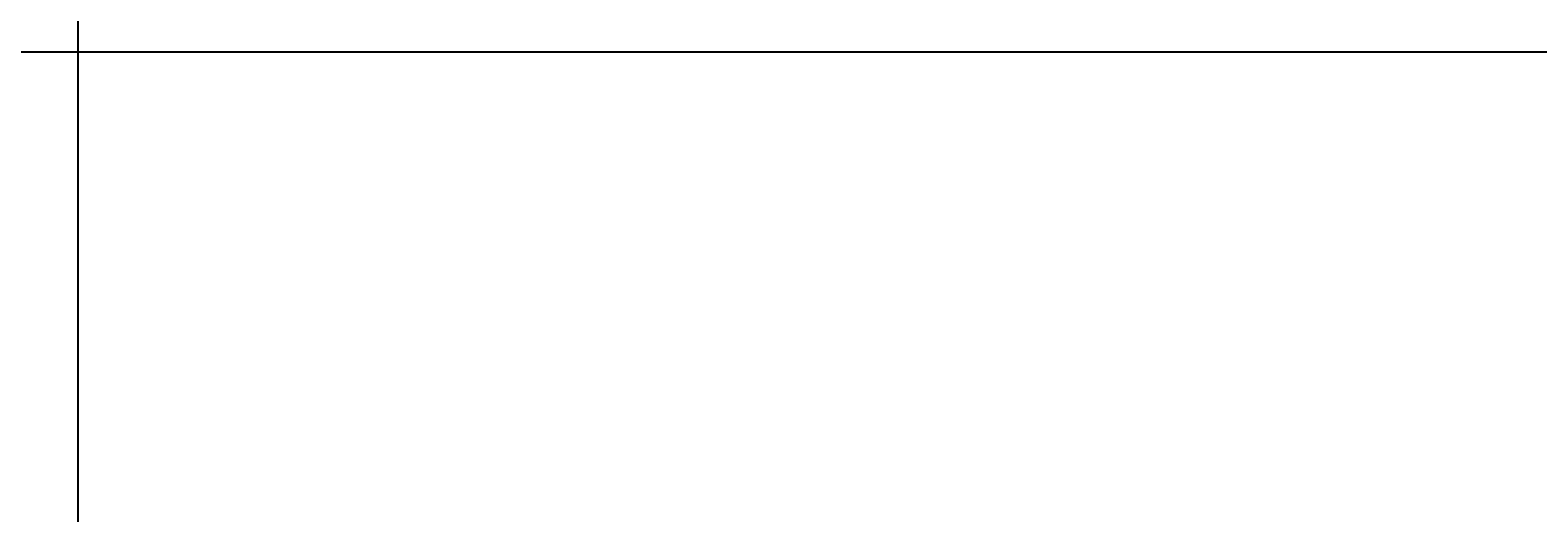
# Model space of a CAD drawing. Units: inches. Extents: x 35362 to 73946, y 43607 to 67532.
# Tile 98 of 134: x 50119 to 50761, y 49064 to 49269. Entities that reach past the tile are written whole.
import ezdxf

# ---------------------------------------------------------------- set-up
doc = ezdxf.new("R2010")
doc.units = ezdxf.units.IN
doc.header["$MEASUREMENT"] = 0
doc.layers.add('A-ANNO-DIMS', color=2, linetype='Continuous', lineweight=18)
doc.styles.get("Standard").update_dxf_attribs({"font": 'arial.ttf'})
doc.dimstyles.get("Standard").update_dxf_attribs({"dimtxt": 0.18, "dimasz": 0.18, "dimexe": 0.18, "dimexo": 0.0625, "dimgap": 0.09, "dimtad": 0, "dimtih": 1, "dimtoh": 1, "dimdec": 4, "dimzin": 0, "dimdsep": 46, "dimtxsty": 'Standard', "dimcen": 0.09, "dimadec": 0, "dimazin": 0, "dimtfac": 1, "dimtdec": 4, "dimtofl": 0, "dimtmove": 0, "dimatfit": 3, "dimfxl": 1, "dimtolj": 1, "dimtzin": 0, "dimarcsym": 0})

# ---------------------------------------------------------------- blocks, each defined once
blk = doc.blocks.new('*D11')
at = {"layer": 'A-ANNO-DIMS', "color": 0, "lineweight": -2, "transparency": 16777216}
for p, q in [((47978.66, 56028.77), (47978.66, 43606.68)), ((53109.76, 56028.77), (53109.76, 43606.68)), ((47978.84, 43606.86), (50543.87, 43606.86)), ((53109.58, 43606.86), (50544.55, 43606.86))]:
    blk.add_line(p, q, dxfattribs=at)
at = {"layer": 'A-ANNO-DIMS', "color": 0, "transparency": 16777216}
for points in [[(47978.84, 43606.89), (47978.84, 43606.83), (47978.66, 43606.86)], [(53109.58, 43606.89), (53109.58, 43606.83), (53109.76, 43606.86)]]:
    blk.add_solid(points, dxfattribs=at)
at = {"layer": 'Defpoints', "color": 0, "transparency": 16777216}
for p in [(47978.66, 56028.84), (53109.76, 56028.84), (53109.76, 43606.86)]:
    blk.add_point(p, dxfattribs=at)
at = {"layer": 'A-ANNO-DIMS', "color": 0, "transparency": 16777216, "insert": (50544.21, 43606.86), "char_height": 0.18, "attachment_point": 5}
blk.add_mtext('\\A1;5131', dxfattribs=at)
blk = doc.blocks.new('*D13')
at = {"layer": 'A-ANNO-DIMS', "color": 0, "lineweight": -2, "transparency": 16777216}
for p, q in [((48373.49, 51694.02), (48373.49, 43606.68)), ((51029.04, 51694.02), (51029.04, 43606.68)), ((48373.67, 43606.86), (49700.8, 43606.86)), ((51028.86, 43606.86), (49701.73, 43606.86))]:
    blk.add_line(p, q, dxfattribs=at)
at = {"layer": 'A-ANNO-DIMS', "color": 0, "transparency": 16777216}
for points in [[(48373.67, 43606.89), (48373.67, 43606.83), (48373.49, 43606.86)], [(51028.86, 43606.89), (51028.86, 43606.83), (51029.04, 43606.86)]]:
    blk.add_solid(points, dxfattribs=at)
at = {"layer": 'Defpoints', "color": 0, "transparency": 16777216}
for p in [(48373.49, 51694.09), (51029.04, 51694.09), (51029.04, 43606.86)]:
    blk.add_point(p, dxfattribs=at)
at = {"layer": 'A-ANNO-DIMS', "color": 0, "transparency": 16777216, "insert": (49701.27, 43606.86), "char_height": 0.18, "attachment_point": 5}
blk.add_mtext('\\A1;2655.6', dxfattribs=at)
blk = doc.blocks.new('*D17')
at = {"layer": 'A-ANNO-DIMS', "color": 0, "lineweight": -2, "transparency": 16777216}
for p, q in [((49923.31, 61293.22), (49923.31, 43606.68)), ((51913.93, 61293.22), (51913.93, 43606.68)), ((49923.49, 43606.86), (50918.16, 43606.86)), ((51913.75, 43606.86), (50919.07, 43606.86))]:
    blk.add_line(p, q, dxfattribs=at)
at = {"layer": 'A-ANNO-DIMS', "color": 0, "transparency": 16777216}
for points in [[(49923.49, 43606.89), (49923.49, 43606.83), (49923.31, 43606.86)], [(51913.75, 43606.89), (51913.75, 43606.83), (51913.93, 43606.86)]]:
    blk.add_solid(points, dxfattribs=at)
at = {"layer": 'Defpoints', "color": 0, "transparency": 16777216}
for p in [(49923.31, 61293.29), (51913.93, 61293.29), (51913.93, 43606.86)]:
    blk.add_point(p, dxfattribs=at)
at = {"layer": 'A-ANNO-DIMS', "color": 0, "transparency": 16777216, "insert": (50918.62, 43606.86), "char_height": 0.18, "attachment_point": 5}
blk.add_mtext('\\A1;1990.6', dxfattribs=at)
blk = doc.blocks.new('*D67')
at = {"layer": 'A-ANNO-DIMS', "color": 0, "lineweight": -2, "transparency": 16777216}
for p, q in [((56873.54, 53351.53), (35361.77, 53351.53)), ((35361.95, 53351.35), (35361.95, 49400.89)), ((35361.95, 45450.07), (35361.95, 49400.53)), ((53793.58, 45449.89), (35361.77, 45449.89))]:
    blk.add_line(p, q, dxfattribs=at)
at = {"layer": 'A-ANNO-DIMS', "color": 0, "transparency": 16777216}
for points in [[(35361.92, 53351.35), (35361.98, 53351.35), (35361.95, 53351.53)], [(35361.92, 45450.07), (35361.98, 45450.07), (35361.95, 45449.89)]]:
    blk.add_solid(points, dxfattribs=at)
at = {"layer": 'Defpoints', "color": 0, "transparency": 16777216}
for p in [(35361.95, 53351.53), (56873.6, 53351.53), (53793.64, 45449.89)]:
    blk.add_point(p, dxfattribs=at)
at = {"layer": 'A-ANNO-DIMS', "color": 0, "transparency": 16777216, "insert": (35361.95, 49400.71), "char_height": 0.18, "attachment_point": 5}
blk.add_mtext('\\A1;7901.6', dxfattribs=at)
blk = doc.blocks.new('*D84')
at = {"layer": 'A-ANNO-DIMS', "color": 0, "lineweight": -2, "transparency": 16777216}
for p, q in [((55540.23, 49259.94), (35361.77, 49259.94)), ((35361.95, 49259.76), (35361.95, 49115.14)), ((35361.95, 48970.16), (35361.95, 49114.78)), ((55540.23, 48969.98), (35361.77, 48969.98))]:
    blk.add_line(p, q, dxfattribs=at)
at = {"layer": 'A-ANNO-DIMS', "color": 0, "transparency": 16777216}
for points in [[(35361.92, 49259.76), (35361.98, 49259.76), (35361.95, 49259.94)], [(35361.92, 48970.16), (35361.98, 48970.16), (35361.95, 48969.98)]]:
    blk.add_solid(points, dxfattribs=at)
at = {"layer": 'Defpoints', "color": 0, "transparency": 16777216}
for p in [(35361.95, 49259.94), (55540.3, 49259.94), (55540.3, 48969.98)]:
    blk.add_point(p, dxfattribs=at)
at = {"layer": 'A-ANNO-DIMS', "color": 0, "transparency": 16777216, "insert": (35361.95, 49114.96), "char_height": 0.18, "attachment_point": 5}
blk.add_mtext('\\A1;289.96', dxfattribs=at)
blk = doc.blocks.new('*D86')
at = {"layer": 'A-ANNO-DIMS', "color": 0, "lineweight": -2, "transparency": 16777216}
for p, q in [((51285.53, 49320.08), (35361.77, 49320.08)), ((35361.95, 49319.9), (35361.95, 49120.26)), ((35361.95, 48920.26), (35361.95, 49119.9)), ((51285.53, 48920.08), (35361.77, 48920.08))]:
    blk.add_line(p, q, dxfattribs=at)
at = {"layer": 'A-ANNO-DIMS', "color": 0, "transparency": 16777216}
for points in [[(35361.92, 49319.9), (35361.98, 49319.9), (35361.95, 49320.08)], [(35361.92, 48920.26), (35361.98, 48920.26), (35361.95, 48920.08)]]:
    blk.add_solid(points, dxfattribs=at)
at = {"layer": 'Defpoints', "color": 0, "transparency": 16777216}
for p in [(35361.95, 49320.08), (51285.59, 49320.08), (51285.59, 48920.08)]:
    blk.add_point(p, dxfattribs=at)
at = {"layer": 'A-ANNO-DIMS', "color": 0, "transparency": 16777216, "insert": (35361.95, 49120.08), "char_height": 0.18, "attachment_point": 5}
blk.add_mtext('\\A1;400.0', dxfattribs=at)
blk = doc.blocks.new('*D107')
at = {"layer": 'A-ANNO-DIMS', "color": 0, "lineweight": -2, "transparency": 16777216}
for p, q in [((50139.56, 59850.01), (50139.56, 43606.68)), ((51320.81, 59850.01), (51320.81, 43606.68)), ((50139.74, 43606.86), (50729.73, 43606.86)), ((51320.63, 43606.86), (50730.64, 43606.86))]:
    blk.add_line(p, q, dxfattribs=at)
at = {"layer": 'A-ANNO-DIMS', "color": 0, "transparency": 16777216}
for points in [[(50139.74, 43606.89), (50139.74, 43606.83), (50139.56, 43606.86)], [(51320.63, 43606.89), (51320.63, 43606.83), (51320.81, 43606.86)]]:
    blk.add_solid(points, dxfattribs=at)
at = {"layer": 'Defpoints', "color": 0, "transparency": 16777216}
for p in [(50139.56, 59850.08), (51320.81, 59850.08), (51320.81, 43606.86)]:
    blk.add_point(p, dxfattribs=at)
at = {"layer": 'A-ANNO-DIMS', "color": 0, "transparency": 16777216, "insert": (50730.19, 43606.86), "char_height": 0.18, "attachment_point": 5}
blk.add_mtext('\\A1;1181.3', dxfattribs=at)

msp = doc.modelspace()

# ---------------------------------------------------------------- dimensions: what is measured, and where the dimension line sits
at = {"layer": 'A-ANNO-DIMS'}
for base, p1, p2, override, picture, middle in [((51913.931, 43606.859), (49923.307, 61293.286), (51913.931, 61293.286), {"dimdec": 1, "dimlfac": 1, "dimrnd": 0, "dimzin": 0, "dimdsep": 46, "dimlunit": 2}, '*D17', (50918.619, 43606.859)), ((51320.8133, 43606.859), (50139.5627, 59850.0769), (51320.8133, 59850.0769), {"dimdec": 1, "dimlfac": 1, "dimrnd": 0, "dimzin": 0, "dimdsep": 46, "dimlunit": 2}, '*D107', (50730.188, 43606.859)), ((53109.76, 43606.859), (47978.665, 56028.836), (53109.76, 56028.836), {"dimdec": 0, "dimlfac": 1, "dimrnd": 0, "dimzin": 0, "dimdsep": 46, "dimlunit": 2}, '*D11', (50544.212, 43606.859)), ((51029.043, 43606.859), (48373.492, 51694.087), (51029.043, 51694.087), {"dimdec": 1, "dimlfac": 1, "dimrnd": 0, "dimzin": 0, "dimdsep": 46, "dimlunit": 2}, '*D13', (49701.267, 43606.859))]:
    dim = msp.add_linear_dim(base=base, p1=p1, p2=p2, dimstyle='Standard', override=override, dxfattribs=at)
    dim.commit()
    dim.dimension.update_dxf_attribs({"geometry": picture, "text_midpoint": middle})
for base, p1, p2, override, picture, middle in [((35361.949, 53351.529), (53793.638, 45449.894), (56873.602, 53351.529), {"dimdec": 1, "dimlfac": 1, "dimrnd": 0, "dimzin": 0, "dimdsep": 46, "dimlunit": 2}, '*D67', (35361.949, 49400.712)), ((35361.949, 49320.079), (51285.595, 48920.079), (51285.595, 49320.079), {"dimdec": 1, "dimlfac": 1, "dimrnd": 0, "dimzin": 0, "dimdsep": 46, "dimlunit": 2}, '*D86', (35361.949, 49120.079)), ((35361.9491, 49259.9353), (55540.2972, 48969.9796), (55540.2972, 49259.9353), {"dimdec": 2, "dimlfac": 1, "dimrnd": 0, "dimzin": 0, "dimdsep": 46, "dimlunit": 2}, '*D84', (35361.9491, 49114.9575))]:
    dim = msp.add_linear_dim(base=base, p1=p1, p2=p2, angle=90, dimstyle='Standard', override=override, dxfattribs=at)
    dim.commit()
    dim.dimension.update_dxf_attribs({"geometry": picture, "text_midpoint": middle})

doc.saveas('drawing.dxf')
